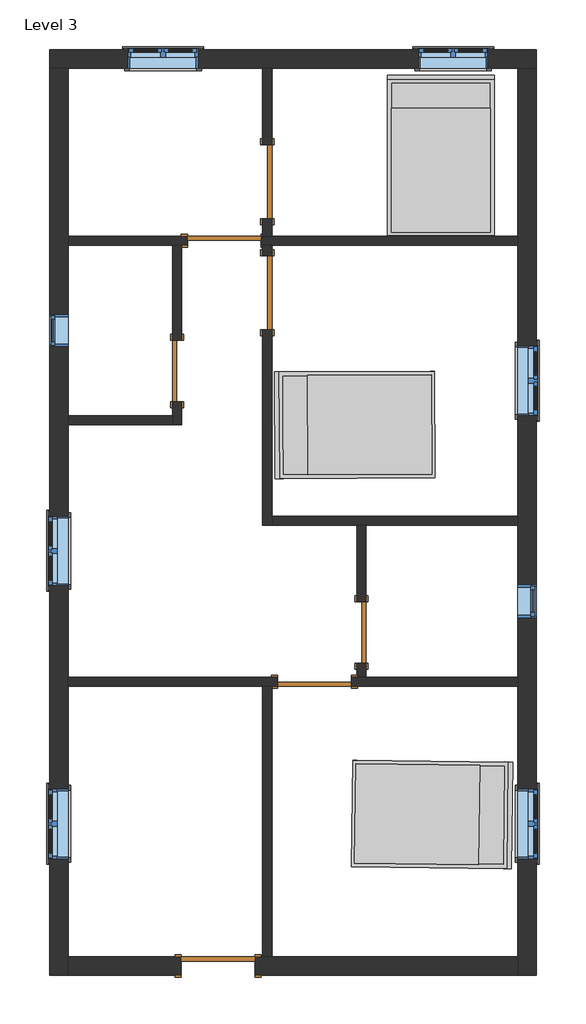
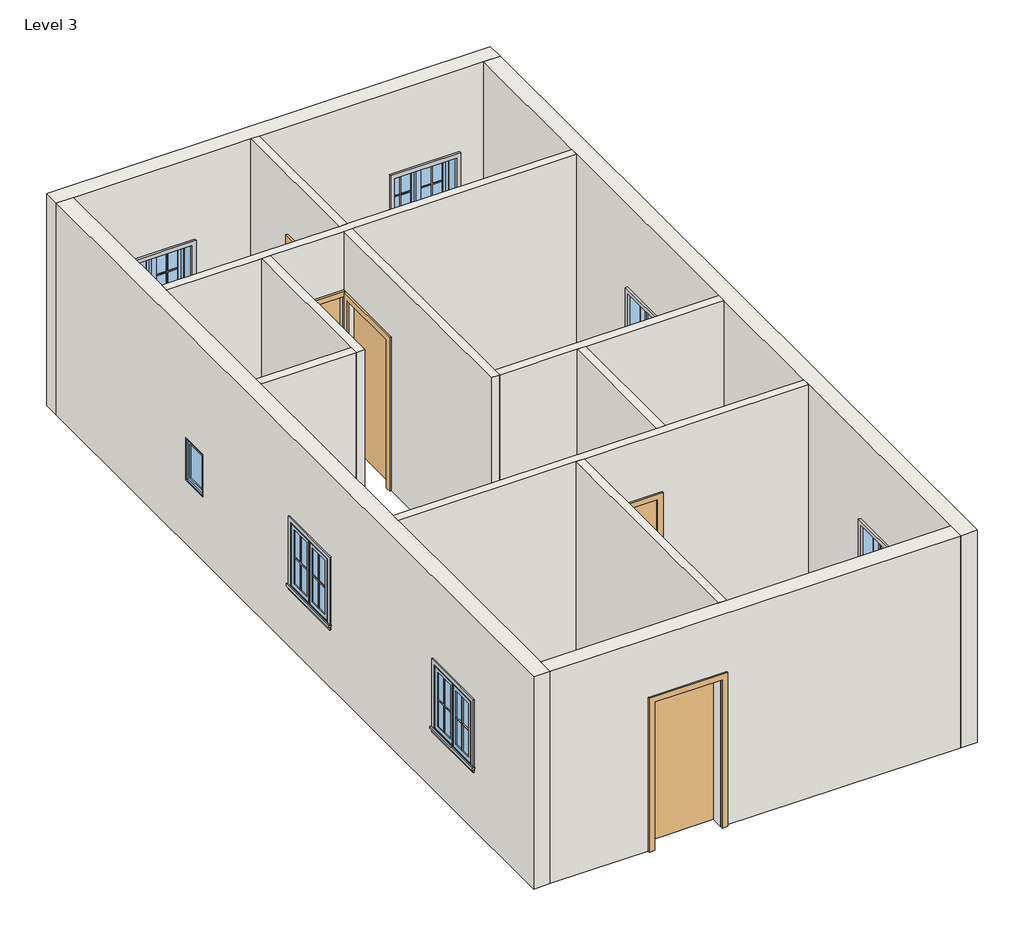
# One storey, incomplete: 24 proxies, 12 walls, 8 windows, 7 doors, 3 furniture elements.
"""IFC4 building model written with IfcOpenShell, lengths in millimetres."""

from ifc_helpers import new_model, si_unit, frame, origin, place, context, project, spatial, polyline, outline, extrude, faceted_brep, transform, mapped, element, save
from components import muntin_pattern_2x2_muntin_pattern_2x2_b3fe6957, muntin_pattern_2x2_muntin_pattern_2x2_3e0ecaf2, trim_window_exterior_flat_with_sill_41619996, trim_window_interior_flat_picture_frame_51c85655, door_d8f5dbb5, door_f2b275c1, door_e5f9f3c4, door_305aa2a5, door_0ca8825f, bed_17739_bed_17739_15c61121, window_aa618e30, window_339605e1

model = new_model("IFC4")

# Units and contexts
model_context = context("Model", 3, world=origin())
ifc_project = project(units=[si_unit("LENGTHUNIT", "METRE", prefix="MILLI")], contexts=[model_context])

# Site, building, storey
site = spatial("IfcSite", under=ifc_project)
building = spatial("IfcBuilding", under=site)
storey = spatial("IfcBuildingStorey", under=building, Name="Level 3", Elevation=3200.4)

# Proxies
placement = place(None, origin())
muntin_pattern_2x2_muntin_pattern_2x2_shape = muntin_pattern_2x2_muntin_pattern_2x2_b3fe6957(model_context)
element("IfcBuildingElementProxy", 1, Name="Muntin Pattern_2x2 : Muntin Pattern_2x2", ObjectType="Muntin Pattern_2x2 : Muntin Pattern_2x2", at=placement, inside=storey, context=model_context, shape_type="MappedRepresentation", body=[
    mapped(muntin_pattern_2x2_muntin_pattern_2x2_shape, transform((517.9959916, 6415.1185985, 4184.65), x_axis=(1.0, 0.0, 0.0), y_axis=(0.0, 1.0, 0.0), z_axis=(0.0, 0.0, 1.0))),
])
element("IfcBuildingElementProxy", 2, Name="Muntin Pattern_2x2 : Muntin Pattern_2x2", ObjectType="Muntin Pattern_2x2 : Muntin Pattern_2x2", at=placement, inside=storey, context=model_context, shape_type="MappedRepresentation", body=[
    mapped(muntin_pattern_2x2_muntin_pattern_2x2_shape, transform((-3079.2790084, 6415.1185985, 4184.65), x_axis=(1.0, 0.0, 0.0), y_axis=(0.0, 1.0, 0.0), z_axis=(0.0, 0.0, 1.0))),
])
element("IfcBuildingElementProxy", 3, Name="Muntin Pattern_2x2 : Muntin Pattern_2x2", ObjectType="Muntin Pattern_2x2 : Muntin Pattern_2x2", at=placement, inside=storey, context=model_context, shape_type="MappedRepresentation", body=[
    mapped(muntin_pattern_2x2_muntin_pattern_2x2_shape, transform((1751.4834916, 2536.8560985, 4184.65), x_axis=(0.0, -1.0, 0.0), y_axis=(1.0, 0.0, 0.0), z_axis=(0.0, 0.0, 1.0))),
])
element("IfcBuildingElementProxy", 4, Name="Muntin Pattern_2x2 : Muntin Pattern_2x2", ObjectType="Muntin Pattern_2x2 : Muntin Pattern_2x2", at=placement, inside=storey, context=model_context, shape_type="MappedRepresentation", body=[
    mapped(muntin_pattern_2x2_muntin_pattern_2x2_shape, transform((-4261.9665084, 0.0310985, 4184.65), x_axis=(0.0, 1.0, 0.0), y_axis=(-1.0, 0.0, 0.0), z_axis=(0.0, 0.0, 1.0))),
])
element("IfcBuildingElementProxy", 5, Name="Muntin Pattern_2x2 : Muntin Pattern_2x2", ObjectType="Muntin Pattern_2x2 : Muntin Pattern_2x2", at=placement, inside=storey, context=model_context, shape_type="MappedRepresentation", body=[
    mapped(muntin_pattern_2x2_muntin_pattern_2x2_shape, transform((-4261.9665084, -3381.3439015, 4184.65), x_axis=(0.0, 1.0, 0.0), y_axis=(-1.0, 0.0, 0.0), z_axis=(0.0, 0.0, 1.0))),
])
element("IfcBuildingElementProxy", 6, Name="Muntin Pattern_2x2 : Muntin Pattern_2x2", ObjectType="Muntin Pattern_2x2 : Muntin Pattern_2x2", at=placement, inside=storey, context=model_context, shape_type="MappedRepresentation", body=[
    mapped(muntin_pattern_2x2_muntin_pattern_2x2_shape, transform((1751.4834916, -2952.7189015, 4184.65), x_axis=(0.0, -1.0, 0.0), y_axis=(1.0, 0.0, 0.0), z_axis=(0.0, 0.0, 1.0))),
])
muntin_pattern_2x2_muntin_pattern_2x2_2_shape = muntin_pattern_2x2_muntin_pattern_2x2_3e0ecaf2(model_context)
element("IfcBuildingElementProxy", 7, Name="Muntin Pattern_2x2 : Muntin Pattern_2x2", ObjectType="Muntin Pattern_2x2 : Muntin Pattern_2x2", at=placement, inside=storey, context=model_context, shape_type="MappedRepresentation", body=[
    mapped(muntin_pattern_2x2_muntin_pattern_2x2_2_shape, transform((946.6209916, 6415.1185985, 4184.65), x_axis=(-1.0, 0.0, 0.0), y_axis=(0.0, -1.0, 0.0), z_axis=(0.0, 0.0, 1.0))),
])
element("IfcBuildingElementProxy", 8, Name="Muntin Pattern_2x2 : Muntin Pattern_2x2", ObjectType="Muntin Pattern_2x2 : Muntin Pattern_2x2", at=placement, inside=storey, context=model_context, shape_type="MappedRepresentation", body=[
    mapped(muntin_pattern_2x2_muntin_pattern_2x2_2_shape, transform((-2650.6540084, 6415.1185985, 4184.65), x_axis=(-1.0, 0.0, 0.0), y_axis=(0.0, -1.0, 0.0), z_axis=(0.0, 0.0, 1.0))),
])
element("IfcBuildingElementProxy", 9, Name="Muntin Pattern_2x2 : Muntin Pattern_2x2", ObjectType="Muntin Pattern_2x2 : Muntin Pattern_2x2", at=placement, inside=storey, context=model_context, shape_type="MappedRepresentation", body=[
    mapped(muntin_pattern_2x2_muntin_pattern_2x2_2_shape, transform((1751.4834916, 2108.2310985, 4184.65), x_axis=(0.0, 1.0, 0.0), y_axis=(-1.0, 0.0, 0.0), z_axis=(0.0, 0.0, 1.0))),
])
element("IfcBuildingElementProxy", 10, Name="Muntin Pattern_2x2 : Muntin Pattern_2x2", ObjectType="Muntin Pattern_2x2 : Muntin Pattern_2x2", at=placement, inside=storey, context=model_context, shape_type="MappedRepresentation", body=[
    mapped(muntin_pattern_2x2_muntin_pattern_2x2_2_shape, transform((-4261.9665084, 428.6560985, 4184.65), x_axis=(0.0, -1.0, 0.0), y_axis=(1.0, 0.0, 0.0), z_axis=(0.0, 0.0, 1.0))),
])
element("IfcBuildingElementProxy", 11, Name="Muntin Pattern_2x2 : Muntin Pattern_2x2", ObjectType="Muntin Pattern_2x2 : Muntin Pattern_2x2", at=placement, inside=storey, context=model_context, shape_type="MappedRepresentation", body=[
    mapped(muntin_pattern_2x2_muntin_pattern_2x2_2_shape, transform((-4261.9665084, -2952.7189015, 4184.65), x_axis=(0.0, -1.0, 0.0), y_axis=(1.0, 0.0, 0.0), z_axis=(0.0, 0.0, 1.0))),
])
element("IfcBuildingElementProxy", 12, Name="Muntin Pattern_2x2 : Muntin Pattern_2x2", ObjectType="Muntin Pattern_2x2 : Muntin Pattern_2x2", at=placement, inside=storey, context=model_context, shape_type="MappedRepresentation", body=[
    mapped(muntin_pattern_2x2_muntin_pattern_2x2_2_shape, transform((1751.4834916, -3381.3439015, 4184.65), x_axis=(0.0, 1.0, 0.0), y_axis=(-1.0, 0.0, 0.0), z_axis=(0.0, 0.0, 1.0))),
])
trim_window_exterior_flat_with_sill_shape = trim_window_exterior_flat_with_sill_41619996(model_context)
element("IfcBuildingElementProxy", 13, Name="Trim-Window-Exterior-Flat : with Sill", ObjectType="Trim-Window-Exterior-Flat : with Sill", at=placement, inside=storey, context=model_context, shape_type="MappedRepresentation", body=[
    mapped(trim_window_exterior_flat_with_sill_shape, transform((732.3084916, 6424.6435985, 5029.2), x_axis=(-1.0, 0.0, 0.0), y_axis=(0.0, 0.0, 1.0), z_axis=(0.0, 1.0, 0.0))),
])
element("IfcBuildingElementProxy", 14, Name="Trim-Window-Exterior-Flat : with Sill", ObjectType="Trim-Window-Exterior-Flat : with Sill", at=placement, inside=storey, context=model_context, shape_type="MappedRepresentation", body=[
    mapped(trim_window_exterior_flat_with_sill_shape, transform((-2864.9665084, 6424.6435985, 5029.2), x_axis=(-1.0, 0.0, 0.0), y_axis=(0.0, 0.0, 1.0), z_axis=(0.0, 1.0, 0.0))),
])
element("IfcBuildingElementProxy", 15, Name="Trim-Window-Exterior-Flat : with Sill", ObjectType="Trim-Window-Exterior-Flat : with Sill", at=placement, inside=storey, context=model_context, shape_type="MappedRepresentation", body=[
    mapped(trim_window_exterior_flat_with_sill_shape, transform((1761.0084916, 2322.5435985, 5029.2), x_axis=(0.0, 1.0, 0.0), y_axis=(0.0, 0.0, 1.0), z_axis=(1.0, 0.0, 0.0))),
])
element("IfcBuildingElementProxy", 16, Name="Trim-Window-Exterior-Flat : with Sill", ObjectType="Trim-Window-Exterior-Flat : with Sill", at=placement, inside=storey, context=model_context, shape_type="MappedRepresentation", body=[
    mapped(trim_window_exterior_flat_with_sill_shape, transform((-4271.4915084, 214.3435985, 5029.2), x_axis=(0.0, -1.0, 0.0), y_axis=(0.0, 0.0, 1.0), z_axis=(-1.0, 0.0, 0.0))),
])
element("IfcBuildingElementProxy", 17, Name="Trim-Window-Exterior-Flat : with Sill", ObjectType="Trim-Window-Exterior-Flat : with Sill", at=placement, inside=storey, context=model_context, shape_type="MappedRepresentation", body=[
    mapped(trim_window_exterior_flat_with_sill_shape, transform((-4271.4915084, -3167.0314015, 5029.2), x_axis=(0.0, -1.0, 0.0), y_axis=(0.0, 0.0, 1.0), z_axis=(-1.0, 0.0, 0.0))),
])
element("IfcBuildingElementProxy", 18, Name="Trim-Window-Exterior-Flat : with Sill", ObjectType="Trim-Window-Exterior-Flat : with Sill", at=placement, inside=storey, context=model_context, shape_type="MappedRepresentation", body=[
    mapped(trim_window_exterior_flat_with_sill_shape, transform((1761.0084916, -3167.0314015, 5029.2), x_axis=(0.0, 1.0, 0.0), y_axis=(0.0, 0.0, 1.0), z_axis=(1.0, 0.0, 0.0))),
])
trim_window_interior_flat_picture_frame_shape = trim_window_interior_flat_picture_frame_51c85655(model_context)
element("IfcBuildingElementProxy", 19, Name="Trim-Window-Interior-Flat : Picture Frame", ObjectType="Trim-Window-Interior-Flat : Picture Frame", at=placement, inside=storey, context=model_context, shape_type="MappedRepresentation", body=[
    mapped(trim_window_interior_flat_picture_frame_shape, transform((732.3084916, 6196.0435985, 5029.2), x_axis=(1.0, 0.0, 0.0), y_axis=(0.0, 0.0, 1.0), z_axis=(0.0, -1.0, 0.0))),
])
element("IfcBuildingElementProxy", 20, Name="Trim-Window-Interior-Flat : Picture Frame", ObjectType="Trim-Window-Interior-Flat : Picture Frame", at=placement, inside=storey, context=model_context, shape_type="MappedRepresentation", body=[
    mapped(trim_window_interior_flat_picture_frame_shape, transform((-2864.9665084, 6196.0435985, 5029.2), x_axis=(1.0, 0.0, 0.0), y_axis=(0.0, 0.0, 1.0), z_axis=(0.0, -1.0, 0.0))),
])
element("IfcBuildingElementProxy", 21, Name="Trim-Window-Interior-Flat : Picture Frame", ObjectType="Trim-Window-Interior-Flat : Picture Frame", at=placement, inside=storey, context=model_context, shape_type="MappedRepresentation", body=[
    mapped(trim_window_interior_flat_picture_frame_shape, transform((1532.4084916, 2322.5435985, 5029.2), x_axis=(0.0, -1.0, 0.0), y_axis=(0.0, 0.0, 1.0), z_axis=(-1.0, 0.0, 0.0))),
])
element("IfcBuildingElementProxy", 22, Name="Trim-Window-Interior-Flat : Picture Frame", ObjectType="Trim-Window-Interior-Flat : Picture Frame", at=placement, inside=storey, context=model_context, shape_type="MappedRepresentation", body=[
    mapped(trim_window_interior_flat_picture_frame_shape, transform((-4042.8915084, 214.3435985, 5029.2), x_axis=(0.0, 1.0, 0.0), y_axis=(0.0, 0.0, 1.0), z_axis=(1.0, 0.0, 0.0))),
])
element("IfcBuildingElementProxy", 23, Name="Trim-Window-Interior-Flat : Picture Frame", ObjectType="Trim-Window-Interior-Flat : Picture Frame", at=placement, inside=storey, context=model_context, shape_type="MappedRepresentation", body=[
    mapped(trim_window_interior_flat_picture_frame_shape, transform((-4042.8915084, -3167.0314015, 5029.2), x_axis=(0.0, 1.0, 0.0), y_axis=(0.0, 0.0, 1.0), z_axis=(1.0, 0.0, 0.0))),
])
element("IfcBuildingElementProxy", 24, Name="Trim-Window-Interior-Flat : Picture Frame", ObjectType="Trim-Window-Interior-Flat : Picture Frame", at=placement, inside=storey, context=model_context, shape_type="MappedRepresentation", body=[
    mapped(trim_window_interior_flat_picture_frame_shape, transform((1532.4084916, -3167.0314015, 5029.2), x_axis=(0.0, -1.0, 0.0), y_axis=(0.0, 0.0, 1.0), z_axis=(-1.0, 0.0, 0.0))),
])

# Doors
door_shape = door_d8f5dbb5(model_context)
element("IfcDoor", 25, ObjectType="Single-Flush : 30\" x 80\"", at=placement, inside=storey, context=model_context, shape_type="MappedRepresentation", body=[
    mapped(door_shape, transform((-404.3415084, -795.3064015, 3200.4), x_axis=(0.0, -1.0, 0.0), y_axis=(1.0, 0.0, 0.0), z_axis=(0.0, 0.0, 1.0))),
])
door_2_shape = door_f2b275c1(model_context)
element("IfcDoor", 26, ObjectType="Single-Flush : 30\" x 80\"", at=placement, inside=storey, context=model_context, shape_type="MappedRepresentation", body=[
    mapped(door_2_shape, transform((-2690.3415084, 2443.1935985, 3200.4), x_axis=(0.0, -1.0, 0.0), y_axis=(1.0, 0.0, 0.0), z_axis=(0.0, 0.0, 1.0))),
])
door_3_shape = door_e5f9f3c4(model_context)
element("IfcDoor", 27, ObjectType="Single-Flush : 36\" x 84\"", at=placement, inside=storey, context=model_context, shape_type="MappedRepresentation", body=[
    mapped(door_3_shape, transform((-2106.1415084, 4056.0935985, 3200.4), x_axis=(1.0, 0.0, 0.0), y_axis=(0.0, 1.0, 0.0), z_axis=(0.0, 0.0, 1.0))),
])
element("IfcDoor", 28, ObjectType="Single-Flush : 36\" x 84\"", at=placement, inside=storey, context=model_context, shape_type="MappedRepresentation", body=[
    mapped(door_3_shape, transform((-1572.7415084, 4786.3435985, 3200.4), x_axis=(0.0, -1.0, 0.0), y_axis=(1.0, 0.0, 0.0), z_axis=(0.0, 0.0, 1.0))),
])
element("IfcDoor", 29, ObjectType="Single-Flush : 36\" x 84\"", at=placement, inside=storey, context=model_context, shape_type="MappedRepresentation", body=[
    mapped(door_3_shape, transform((-988.5415084, -1404.9064015, 3200.4), x_axis=(-1.0, 0.0, 0.0), y_axis=(0.0, -1.0, 0.0), z_axis=(0.0, 0.0, 1.0))),
])
door_4_shape = door_305aa2a5(model_context)
element("IfcDoor", 30, ObjectType="Single-Flush : 36\" x 84\"", at=placement, inside=storey, context=model_context, shape_type="MappedRepresentation", body=[
    mapped(door_4_shape, transform((-1572.7415084, 3414.7435985, 3200.4), x_axis=(0.0, 1.0, 0.0), y_axis=(-1.0, 0.0, 0.0), z_axis=(0.0, 0.0, 1.0))),
])
door_5_shape = door_0ca8825f(model_context)
element("IfcDoor", 31, ObjectType="Single-Flush : 36\" x 84\"", at=placement, inside=storey, context=model_context, shape_type="MappedRepresentation", body=[
    mapped(door_5_shape, transform((-2182.3415084, -4929.1564015, 3200.4), x_axis=(1.0, 0.0, 0.0), y_axis=(0.0, 1.0, 0.0), z_axis=(0.0, 0.0, 1.0))),
])

# Furniture
bed_17739_bed_17739_shape = bed_17739_bed_17739_15c61121(model_context)
element("IfcFurniture", 32, ObjectType="Bed_17739 : Bed_17739", at=placement, inside=storey, context=model_context, shape_type="MappedRepresentation", body=[
    mapped(bed_17739_bed_17739_shape, transform((579.9084916, 5091.1435985, 3200.4), x_axis=(1.0, 0.0, 0.0), y_axis=(0.0, 1.0, 0.0), z_axis=(0.0, 0.0, 1.0))),
])
element("IfcFurniture", 33, ObjectType="Bed_17739 : Bed_17739", at=placement, inside=storey, context=model_context, shape_type="MappedRepresentation", body=[
    mapped(bed_17739_bed_17739_shape, transform((-461.4915084, 1776.4435985, 3200.4), x_axis=(-0.00529598194226197, 0.9999859761893001, 0.0), y_axis=(-0.9999859761893001, -0.00529598194226197, 0.0), z_axis=(0.0, 0.0, 1.0))),
])
element("IfcFurniture", 34, ObjectType="Bed_17739 : Bed_17739", at=placement, inside=storey, context=model_context, shape_type="MappedRepresentation", body=[
    mapped(bed_17739_bed_17739_shape, transform((445.2457081, -3048.1973462, 3200.4), x_axis=(-0.012781947661401841, -0.9999183075701641, 0.0), y_axis=(0.9999183075701641, -0.012781947661401841, 0.0), z_axis=(0.0, 0.0, 1.0))),
])

# Walls
element("IfcWall", 35, ObjectType="WALL4.5\"", at=placement, inside=storey, context=model_context, shape_type="Brep", body=[
    faceted_brep([(-1648.9415084, 3998.9435985, 5334.0), (-1648.9415084, 3998.9435985, 3200.4), (-1629.8915084, 3998.9435985, 3200.4), (-1515.5915084, 3998.9435985, 3200.4), (1532.4084916, 3998.9435985, 3200.4), (1532.4084916, 3998.9435985, 6248.4), (-1515.5915084, 3998.9435985, 6248.4), (-1629.8915084, 3998.9435985, 6248.4), (-2633.1915084, 3998.9435985, 6248.4), (-2747.4915084, 3998.9435985, 6248.4), (-4042.8915084, 3998.9435985, 6248.4), (-4042.8915084, 3998.9435985, 3200.4), (-2747.4915084, 3998.9435985, 3200.4), (-2633.1915084, 3998.9435985, 3200.4), (-2563.3415084, 3998.9435985, 3200.4), (-2563.3415084, 3998.9435985, 5334.0), (1532.4084916, 4113.2435985, 3200.4), (-1515.5915084, 4113.2435985, 3200.4), (-1629.8915084, 4113.2435985, 3200.4), (-1648.9415084, 4113.2435985, 3200.4), (-1648.9415084, 4113.2435985, 5334.0), (-2563.3415084, 4113.2435985, 5334.0), (-2563.3415084, 4113.2435985, 3200.4), (-4042.8915084, 4113.2435985, 3200.4), (-4042.8915084, 4113.2435985, 6248.4), (-1629.8915084, 4113.2435985, 6248.4), (-1515.5915084, 4113.2435985, 6248.4), (1532.4084916, 4113.2435985, 6248.4)], [[[0, 1, 2, 3, 4, 5, 6, 7, 8, 9, 10, 11, 12, 13, 14, 15]], [[16, 17, 18, 19, 20, 21, 22, 23, 24, 25, 26, 27]], [[4, 3, 2, 1, 19, 18, 17, 16]], [[14, 13, 12, 11, 23, 22]], [[5, 4, 16, 27]], [[11, 10, 24, 23]], [[20, 19, 1, 0]], [[21, 20, 0, 15]], [[22, 21, 15, 14]], [[10, 9, 8, 7, 6, 5, 27, 26, 25, 24]]]),
])
element("IfcWall", 36, ObjectType="WALL4.5\"", at=placement, inside=storey, context=model_context, shape_type="Brep", body=[
    faceted_brep([(-1629.8915084, 6196.0435985, 6248.4), (-1629.8915084, 6196.0435985, 3200.4), (-1629.8915084, 5243.5435985, 3200.4), (-1629.8915084, 5243.5435985, 5334.0), (-1629.8915084, 4329.1435985, 5334.0), (-1629.8915084, 4329.1435985, 3200.4), (-1629.8915084, 4113.2435985, 3200.4), (-1629.8915084, 4113.2435985, 6248.4), (-1515.5915084, 6196.0435985, 3200.4), (-1515.5915084, 6196.0435985, 6248.4), (-1515.5915084, 4113.2435985, 6248.4), (-1515.5915084, 4113.2435985, 3200.4), (-1515.5915084, 4329.1435985, 3200.4), (-1515.5915084, 4329.1435985, 5334.0), (-1515.5915084, 5243.5435985, 5334.0), (-1515.5915084, 5243.5435985, 3200.4)], [[[0, 1, 2, 3, 4, 5, 6, 7]], [[8, 9, 10, 11, 12, 13, 14, 15]], [[1, 8, 15, 2]], [[5, 12, 11, 6]], [[1, 0, 9, 8]], [[7, 6, 11, 10]], [[13, 12, 5, 4]], [[14, 13, 4, 3]], [[15, 14, 3, 2]], [[9, 0, 7, 10]]]),
    faceted_brep([(-1629.8915084, 531.8435985, 3200.4), (-1629.8915084, 531.8435985, 6248.4), (-1629.8915084, 3998.9435985, 6248.4), (-1629.8915084, 3998.9435985, 3200.4), (-1629.8915084, 3871.9435985, 3200.4), (-1629.8915084, 3871.9435985, 5334.0), (-1629.8915084, 2957.5435985, 5334.0), (-1629.8915084, 2957.5435985, 3200.4), (-1515.5915084, 531.8435985, 6248.4), (-1515.5915084, 531.8435985, 3200.4), (-1515.5915084, 646.1435985, 3200.4), (-1515.5915084, 2957.5435985, 3200.4), (-1515.5915084, 2957.5435985, 5334.0), (-1515.5915084, 3871.9435985, 5334.0), (-1515.5915084, 3871.9435985, 3200.4), (-1515.5915084, 3998.9435985, 3200.4), (-1515.5915084, 3998.9435985, 6248.4), (-1515.5915084, 646.1435985, 6248.4)], [[[0, 1, 2, 3, 4, 5, 6, 7]], [[8, 9, 10, 11, 12, 13, 14, 15, 16, 17]], [[9, 0, 7, 11, 10]], [[14, 4, 3, 15]], [[3, 2, 16, 15]], [[1, 0, 9, 8]], [[5, 4, 14, 13]], [[6, 5, 13, 12]], [[7, 6, 12, 11]], [[1, 8, 17, 16, 2]]]),
])
element("IfcWall", 37, ObjectType="WALL4.5\"", at=placement, inside=storey, context=model_context, shape_type="Brep", body=[
    faceted_brep([(-1515.5915084, 531.8435985, 3200.4), (-461.4915084, 531.8435985, 3200.4), (-347.1915084, 531.8435985, 3200.4), (1532.4084916, 531.8435985, 3200.4), (1532.4084916, 531.8435985, 6248.4), (-347.1915084, 531.8435985, 6248.4), (-461.4915084, 531.8435985, 6248.4), (-1515.5915084, 531.8435985, 6248.4), (-1515.5915084, 646.1435985, 3200.4), (-1515.5915084, 646.1435985, 6248.4), (1532.4084916, 646.1435985, 6248.4), (1532.4084916, 646.1435985, 3200.4)], [[[0, 1, 2, 3, 4, 5, 6, 7]], [[8, 9, 10, 11]], [[3, 2, 1, 0, 8, 11]], [[0, 7, 9, 8]], [[4, 3, 11, 10]], [[7, 6, 5, 4, 10, 9]]]),
])
element("IfcWall", 38, ObjectType="WALL4.5\"", at=placement, inside=storey, context=model_context, shape_type="Brep", body=[
    faceted_brep([(-2747.4915084, 2062.1935985, 5232.4), (-2747.4915084, 2062.1935985, 3200.4), (-2747.4915084, 1890.7435985, 3200.4), (-2747.4915084, 1776.4435985, 3200.4), (-2747.4915084, 1776.4435985, 6248.4), (-2747.4915084, 1890.7435985, 6248.4), (-2747.4915084, 3998.9435985, 6248.4), (-2747.4915084, 3998.9435985, 3200.4), (-2747.4915084, 2824.1935985, 3200.4), (-2747.4915084, 2824.1935985, 5232.4), (-2633.1915084, 1776.4435985, 3200.4), (-2633.1915084, 2062.1935985, 3200.4), (-2633.1915084, 2062.1935985, 5232.4), (-2633.1915084, 2824.1935985, 5232.4), (-2633.1915084, 2824.1935985, 3200.4), (-2633.1915084, 3998.9435985, 3200.4), (-2633.1915084, 3998.9435985, 6248.4), (-2633.1915084, 1776.4435985, 6248.4)], [[[0, 1, 2, 3, 4, 5, 6, 7, 8, 9]], [[10, 11, 12, 13, 14, 15, 16, 17]], [[8, 7, 15, 14]], [[3, 2, 1, 11, 10]], [[7, 6, 16, 15]], [[4, 3, 10, 17]], [[12, 11, 1, 0]], [[13, 12, 0, 9]], [[14, 13, 9, 8]], [[6, 5, 4, 17, 16]]]),
])
element("IfcWall", 39, ObjectType="WALL4.5\"", at=placement, inside=storey, context=model_context, shape_type="SweptSolid", body=[
    extrude(outline(polyline([(-2747.4915084, 1776.4435985), (-4042.8915084, 1776.4435985), (-4042.8915084, 1890.7435985), (-2747.4915084, 1890.7435985), (-2747.4915084, 1776.4435985)])), frame((0.0, 0.0, 3200.4), z_axis=(0.0, 0.0, 1.0), x_axis=(1.0, 0.0, 0.0)), (0.0, 0.0, 1.0), 3048.0),
])
element("IfcWall", 40, ObjectType="WALL4.5\"", at=placement, inside=storey, context=model_context, shape_type="SweptSolid", body=[
    extrude(outline(polyline([(-1176.3064015, 5232.4), (-1176.3064015, 3200.4), (-1347.7564015, 3200.4), (-1347.7564015, 6248.4), (531.8435985, 6248.4), (531.8435985, 3200.4), (-414.3064015, 3200.4), (-414.3064015, 5232.4), (-1176.3064015, 5232.4)])), frame((-461.4915084, 0.0, 0.0), z_axis=(1.0, 0.0, 0.0), x_axis=(0.0, 1.0, 0.0)), (0.0, 0.0, 1.0), 114.3),
])
element("IfcWall", 41, ObjectType="WALL4.5\"", at=placement, inside=storey, context=model_context, shape_type="Brep", body=[
    faceted_brep([(-4042.8915084, -1462.0564015, 3200.4), (-1629.8915084, -1462.0564015, 3200.4), (-1515.5915084, -1462.0564015, 3200.4), (-1445.7415084, -1462.0564015, 3200.4), (-1445.7415084, -1462.0564015, 5334.0), (-531.3415084, -1462.0564015, 5334.0), (-531.3415084, -1462.0564015, 3200.4), (1532.4084916, -1462.0564015, 3200.4), (1532.4084916, -1462.0564015, 6248.4), (-1515.5915084, -1462.0564015, 6248.4), (-1629.8915084, -1462.0564015, 6248.4), (-4042.8915084, -1462.0564015, 6248.4), (-1445.7415084, -1347.7564015, 5334.0), (-1445.7415084, -1347.7564015, 3200.4), (-4042.8915084, -1347.7564015, 3200.4), (-4042.8915084, -1347.7564015, 6248.4), (-461.4915084, -1347.7564015, 6248.4), (-347.1915084, -1347.7564015, 6248.4), (1532.4084916, -1347.7564015, 6248.4), (1532.4084916, -1347.7564015, 3200.4), (-347.1915084, -1347.7564015, 3200.4), (-461.4915084, -1347.7564015, 3200.4), (-531.3415084, -1347.7564015, 3200.4), (-531.3415084, -1347.7564015, 5334.0)], [[[0, 1, 2, 3, 4, 5, 6, 7, 8, 9, 10, 11]], [[12, 13, 14, 15, 16, 17, 18, 19, 20, 21, 22, 23]], [[14, 13, 3, 2, 1, 0]], [[22, 21, 20, 19, 7, 6]], [[8, 7, 19, 18]], [[0, 11, 15, 14]], [[4, 3, 13, 12]], [[5, 4, 12, 23]], [[6, 5, 23, 22]], [[11, 10, 9, 8, 18, 17, 16, 15]]]),
])
element("IfcWall", 42, ObjectType="WALL4.5\"", at=placement, inside=storey, context=model_context, shape_type="SweptSolid", body=[
    extrude(outline(polyline([(-1629.8915084, -4814.8564015), (-1629.8915084, -1462.0564015), (-1515.5915084, -1462.0564015), (-1515.5915084, -4814.8564015), (-1629.8915084, -4814.8564015)])), frame((0.0, 0.0, 3200.4), z_axis=(0.0, 0.0, 1.0), x_axis=(1.0, 0.0, 0.0)), (0.0, 0.0, 1.0), 3048.0),
])
element("IfcWall", 43, ObjectType="WALL9\"", at=placement, inside=storey, context=model_context, shape_type="Brep", body=[
    faceted_brep([(-4271.4915084, 6196.0435985, 3200.4), (-4042.8915084, 6196.0435985, 3200.4), (-1629.8915084, 6196.0435985, 3200.4), (-1515.5915084, 6196.0435985, 3200.4), (1532.4084916, 6196.0435985, 3200.4), (1761.0084916, 6196.0435985, 3200.4), (1761.0084916, 6196.0435985, 6248.4), (1532.4084916, 6196.0435985, 6248.4), (-1515.5915084, 6196.0435985, 6248.4), (-1629.8915084, 6196.0435985, 6248.4), (-4042.8915084, 6196.0435985, 6248.4), (-4271.4915084, 6196.0435985, 6248.4), (1164.1084916, 6196.0435985, 5029.2), (1164.1084916, 6196.0435985, 4114.8), (300.5084916, 6196.0435985, 4114.8), (300.5084916, 6196.0435985, 5029.2), (-2433.1665084, 6196.0435985, 5029.2), (-2433.1665084, 6196.0435985, 4114.8), (-3296.7665084, 6196.0435985, 4114.8), (-3296.7665084, 6196.0435985, 5029.2), (-4271.4915084, 6424.6435985, 3200.4), (-4271.4915084, 6424.6435985, 6248.4), (1761.0084916, 6424.6435985, 6248.4), (1761.0084916, 6424.6435985, 3200.4), (1164.1084916, 6424.6435985, 5029.2), (300.5084916, 6424.6435985, 5029.2), (300.5084916, 6424.6435985, 4114.8), (1164.1084916, 6424.6435985, 4114.8), (-2433.1665084, 6424.6435985, 5029.2), (-3296.7665084, 6424.6435985, 5029.2), (-3296.7665084, 6424.6435985, 4114.8), (-2433.1665084, 6424.6435985, 4114.8)], [[[0, 1, 2, 3, 4, 5, 6, 7, 8, 9, 10, 11], [12, 13, 14, 15], [16, 17, 18, 19]], [[20, 21, 22, 23], [24, 25, 26, 27], [28, 29, 30, 31]], [[5, 4, 3, 2, 1, 0, 20, 23]], [[6, 5, 23, 22]], [[0, 11, 21, 20]], [[13, 12, 24, 27]], [[14, 13, 27, 26]], [[15, 14, 26, 25]], [[12, 15, 25, 24]], [[17, 16, 28, 31]], [[18, 17, 31, 30]], [[19, 18, 30, 29]], [[16, 19, 29, 28]], [[11, 10, 9, 8, 7, 6, 22, 21]]]),
])
element("IfcWall", 44, ObjectType="WALL9\"", at=placement, inside=storey, context=model_context, shape_type="Brep", body=[
    faceted_brep([(1532.4084916, 6196.0435985, 3200.4), (1532.4084916, 4113.2435985, 3200.4), (1532.4084916, 3998.9435985, 3200.4), (1532.4084916, 646.1435985, 3200.4), (1532.4084916, 531.8435985, 3200.4), (1532.4084916, -1347.7564015, 3200.4), (1532.4084916, -1462.0564015, 3200.4), (1532.4084916, -4814.8564015, 3200.4), (1532.4084916, -5043.4564015, 3200.4), (1532.4084916, -5043.4564015, 6248.4), (1532.4084916, -4814.8564015, 6248.4), (1532.4084916, -1462.0564015, 6248.4), (1532.4084916, -1347.7564015, 6248.4), (1532.4084916, 531.8435985, 6248.4), (1532.4084916, 646.1435985, 6248.4), (1532.4084916, 3998.9435985, 6248.4), (1532.4084916, 4113.2435985, 6248.4), (1532.4084916, 6196.0435985, 6248.4), (1532.4084916, -611.1564015, 4724.4), (1532.4084916, -611.1564015, 4114.8), (1532.4084916, -204.7564015, 4114.8), (1532.4084916, -204.7564015, 4724.4), (1532.4084916, 1890.7435985, 5029.2), (1532.4084916, 1890.7435985, 4114.8), (1532.4084916, 2754.3435985, 4114.8), (1532.4084916, 2754.3435985, 5029.2), (1532.4084916, -3598.8314015, 5029.2), (1532.4084916, -3598.8314015, 4114.8), (1532.4084916, -2735.2314015, 4114.8), (1532.4084916, -2735.2314015, 5029.2), (1761.0084916, 6196.0435985, 3200.4), (1761.0084916, 6196.0435985, 6248.4), (1761.0084916, -5043.4564015, 6248.4), (1761.0084916, -5043.4564015, 3200.4), (1761.0084916, -611.1564015, 4724.4), (1761.0084916, -204.7564015, 4724.4), (1761.0084916, -204.7564015, 4114.8), (1761.0084916, -611.1564015, 4114.8), (1761.0084916, 1890.7435985, 5029.2), (1761.0084916, 2754.3435985, 5029.2), (1761.0084916, 2754.3435985, 4114.8), (1761.0084916, 1890.7435985, 4114.8), (1761.0084916, -3598.8314015, 5029.2), (1761.0084916, -2735.2314015, 5029.2), (1761.0084916, -2735.2314015, 4114.8), (1761.0084916, -3598.8314015, 4114.8)], [[[0, 1, 2, 3, 4, 5, 6, 7, 8, 9, 10, 11, 12, 13, 14, 15, 16, 17], [18, 19, 20, 21], [22, 23, 24, 25], [26, 27, 28, 29]], [[30, 31, 32, 33], [34, 35, 36, 37], [38, 39, 40, 41], [42, 43, 44, 45]], [[8, 7, 6, 5, 4, 3, 2, 1, 0, 30, 33]], [[0, 17, 31, 30]], [[9, 8, 33, 32]], [[19, 18, 34, 37]], [[20, 19, 37, 36]], [[21, 20, 36, 35]], [[18, 21, 35, 34]], [[23, 22, 38, 41]], [[24, 23, 41, 40]], [[25, 24, 40, 39]], [[22, 25, 39, 38]], [[27, 26, 42, 45]], [[28, 27, 45, 44]], [[29, 28, 44, 43]], [[26, 29, 43, 42]], [[17, 16, 15, 14, 13, 12, 11, 10, 9, 32, 31]]]),
])
element("IfcWall", 45, ObjectType="WALL9\"", at=placement, inside=storey, context=model_context, shape_type="Brep", body=[
    faceted_brep([(-4271.4915084, 6196.0435985, 3200.4), (-4271.4915084, -5043.4564015, 3200.4), (-4271.4915084, -5043.4564015, 6248.4), (-4271.4915084, 6196.0435985, 6248.4), (-4271.4915084, 3148.0435985, 4724.4), (-4271.4915084, 2741.6435985, 4724.4), (-4271.4915084, 2741.6435985, 4114.8), (-4271.4915084, 3148.0435985, 4114.8), (-4271.4915084, 646.1435985, 5029.2), (-4271.4915084, -217.4564015, 5029.2), (-4271.4915084, -217.4564015, 4114.8), (-4271.4915084, 646.1435985, 4114.8), (-4271.4915084, -2735.2314015, 5029.2), (-4271.4915084, -3598.8314015, 5029.2), (-4271.4915084, -3598.8314015, 4114.8), (-4271.4915084, -2735.2314015, 4114.8), (-4042.8915084, 6196.0435985, 3200.4), (-4042.8915084, 6196.0435985, 6248.4), (-4042.8915084, 4113.2435985, 6248.4), (-4042.8915084, 3998.9435985, 6248.4), (-4042.8915084, 1890.7435985, 6248.4), (-4042.8915084, 1776.4435985, 6248.4), (-4042.8915084, -1347.7564015, 6248.4), (-4042.8915084, -1462.0564015, 6248.4), (-4042.8915084, -4814.8564015, 6248.4), (-4042.8915084, -5043.4564015, 6248.4), (-4042.8915084, -5043.4564015, 3200.4), (-4042.8915084, -4814.8564015, 3200.4), (-4042.8915084, -1462.0564015, 3200.4), (-4042.8915084, -1347.7564015, 3200.4), (-4042.8915084, 1776.4435985, 3200.4), (-4042.8915084, 1890.7435985, 3200.4), (-4042.8915084, 3998.9435985, 3200.4), (-4042.8915084, 4113.2435985, 3200.4), (-4042.8915084, 3148.0435985, 4724.4), (-4042.8915084, 3148.0435985, 4114.8), (-4042.8915084, 2741.6435985, 4114.8), (-4042.8915084, 2741.6435985, 4724.4), (-4042.8915084, 646.1435985, 5029.2), (-4042.8915084, 646.1435985, 4114.8), (-4042.8915084, -217.4564015, 4114.8), (-4042.8915084, -217.4564015, 5029.2), (-4042.8915084, -2735.2314015, 5029.2), (-4042.8915084, -2735.2314015, 4114.8), (-4042.8915084, -3598.8314015, 4114.8), (-4042.8915084, -3598.8314015, 5029.2)], [[[0, 1, 2, 3], [4, 5, 6, 7], [8, 9, 10, 11], [12, 13, 14, 15]], [[16, 17, 18, 19, 20, 21, 22, 23, 24, 25, 26, 27, 28, 29, 30, 31, 32, 33], [34, 35, 36, 37], [38, 39, 40, 41], [42, 43, 44, 45]], [[1, 0, 16, 33, 32, 31, 30, 29, 28, 27, 26]], [[0, 3, 17, 16]], [[2, 1, 26, 25]], [[35, 34, 4, 7]], [[36, 35, 7, 6]], [[37, 36, 6, 5]], [[34, 37, 5, 4]], [[39, 38, 8, 11]], [[40, 39, 11, 10]], [[41, 40, 10, 9]], [[38, 41, 9, 8]], [[43, 42, 12, 15]], [[44, 43, 15, 14]], [[45, 44, 14, 13]], [[42, 45, 13, 12]], [[3, 2, 25, 24, 23, 22, 21, 20, 19, 18, 17]]]),
])
element("IfcWall", 46, ObjectType="WALL9\"", at=placement, inside=storey, context=model_context, shape_type="Brep", body=[
    faceted_brep([(-1725.1415084, -5043.4564015, 5334.0), (-1725.1415084, -5043.4564015, 3200.4), (1532.4084916, -5043.4564015, 3200.4), (1532.4084916, -5043.4564015, 6248.4), (-4042.8915084, -5043.4564015, 6248.4), (-4042.8915084, -5043.4564015, 3200.4), (-2639.5415084, -5043.4564015, 3200.4), (-2639.5415084, -5043.4564015, 5334.0), (1532.4084916, -4814.8564015, 3200.4), (-1515.5915084, -4814.8564015, 3200.4), (-1629.8915084, -4814.8564015, 3200.4), (-1725.1415084, -4814.8564015, 3200.4), (-1725.1415084, -4814.8564015, 5334.0), (-2639.5415084, -4814.8564015, 5334.0), (-2639.5415084, -4814.8564015, 3200.4), (-4042.8915084, -4814.8564015, 3200.4), (-4042.8915084, -4814.8564015, 6248.4), (-1629.8915084, -4814.8564015, 6248.4), (-1515.5915084, -4814.8564015, 6248.4), (1532.4084916, -4814.8564015, 6248.4)], [[[0, 1, 2, 3, 4, 5, 6, 7]], [[8, 9, 10, 11, 12, 13, 14, 15, 16, 17, 18, 19]], [[6, 5, 15, 14]], [[2, 1, 11, 10, 9, 8]], [[3, 2, 8, 19]], [[5, 4, 16, 15]], [[12, 11, 1, 0]], [[13, 12, 0, 7]], [[14, 13, 7, 6]], [[4, 3, 19, 18, 17, 16]]]),
])

# Windows
window_shape = window_aa618e30(model_context)
element("IfcWindow", 47, ObjectType="Fixed : 16\" x 24\"", at=placement, inside=storey, context=model_context, shape_type="MappedRepresentation", body=[
    mapped(window_shape, transform((1646.7084916, -446.0564015, 3200.4), x_axis=(0.0, -1.0, 0.0), y_axis=(1.0, 0.0, 0.0), z_axis=(0.0, 0.0, 1.0))),
])
element("IfcWindow", 48, ObjectType="Fixed : 16\" x 24\"", at=placement, inside=storey, context=model_context, shape_type="MappedRepresentation", body=[
    mapped(window_shape, transform((-4157.1915084, 2982.9435985, 3200.4), x_axis=(0.0, 1.0, 0.0), y_axis=(-1.0, 0.0, 0.0), z_axis=(0.0, 0.0, 1.0))),
])
window_2_shape = window_339605e1(model_context)
element("IfcWindow", 49, ObjectType="Window-Casement-Double : 34\" x 36\"", at=placement, inside=storey, context=model_context, shape_type="MappedRepresentation", body=[
    mapped(window_2_shape, transform((732.3084916, 6310.3435985, 3200.4), x_axis=(1.0, 0.0, 0.0), y_axis=(0.0, 1.0, 0.0), z_axis=(0.0, 0.0, 1.0))),
])
element("IfcWindow", 50, ObjectType="Window-Casement-Double : 34\" x 36\"", at=placement, inside=storey, context=model_context, shape_type="MappedRepresentation", body=[
    mapped(window_2_shape, transform((-2864.9665084, 6310.3435985, 3200.4), x_axis=(1.0, 0.0, 0.0), y_axis=(0.0, 1.0, 0.0), z_axis=(0.0, 0.0, 1.0))),
])
element("IfcWindow", 51, ObjectType="Window-Casement-Double : 34\" x 36\"", at=placement, inside=storey, context=model_context, shape_type="MappedRepresentation", body=[
    mapped(window_2_shape, transform((1646.7084916, 2322.5435985, 3200.4), x_axis=(0.0, -1.0, 0.0), y_axis=(1.0, 0.0, 0.0), z_axis=(0.0, 0.0, 1.0))),
])
element("IfcWindow", 52, ObjectType="Window-Casement-Double : 34\" x 36\"", at=placement, inside=storey, context=model_context, shape_type="MappedRepresentation", body=[
    mapped(window_2_shape, transform((-4157.1915084, 214.3435985, 3200.4), x_axis=(0.0, 1.0, 0.0), y_axis=(-1.0, 0.0, 0.0), z_axis=(0.0, 0.0, 1.0))),
])
element("IfcWindow", 53, ObjectType="Window-Casement-Double : 34\" x 36\"", at=placement, inside=storey, context=model_context, shape_type="MappedRepresentation", body=[
    mapped(window_2_shape, transform((-4157.1915084, -3167.0314015, 3200.4), x_axis=(0.0, 1.0, 0.0), y_axis=(-1.0, 0.0, 0.0), z_axis=(0.0, 0.0, 1.0))),
])
element("IfcWindow", 54, ObjectType="Window-Casement-Double : 34\" x 36\"", at=placement, inside=storey, context=model_context, shape_type="MappedRepresentation", body=[
    mapped(window_2_shape, transform((1646.7084916, -3167.0314015, 3200.4), x_axis=(0.0, -1.0, 0.0), y_axis=(1.0, 0.0, 0.0), z_axis=(0.0, 0.0, 1.0))),
])

save(model, "model.ifc")

# Revit data of these elements
# Type "Muntin Pattern_2x2 : Muntin Pattern_2x2"
#   Width [instance default] = 4' - 0"
#   Thickness = 0' - 0 1/2"
#   Height [instance default] = 4' - 0"
#   Distance = 0' - 0 3/4"
#   Interior Material [instance default] = none
#   Exterior Material [instance default] = none
#   Default Elevation = 0
# Type "Trim-Window-Exterior-Flat : with Sill"
#   Trim Width = 0' - 2 1/4"
#   Trim Thickness_Picture Frame = 0' - 1 1/4"
#   Trim Thickness_with Sill = 0' - 0 3/4"
#   Sill Thickness = 0' - 1 1/4"
#   Opening Width [instance default] = 2' - 0"
#   Opening Height [instance default] = 3' - 0"
#   Default Elevation = 4' - 0"
#   Sill = yes
#   Picture Frame = no
#   Trim Material [instance default] = none
# Type "Trim-Window-Interior-Flat : Picture Frame"
#   Trim Thickness_Picture Frame = 0' - 1 1/4"
#   Trim Width = 0' - 2 1/4"
#   Trim Thickness_with Sill = 0' - 0 3/4"
#   Sill Thickness = 0' - 1 1/4"
#   Opening Width [instance default] = 2' - 0"
#   Opening Height [instance default] = 3' - 0"
#   Default Elevation = 4' - 0"
#   Sill = no
#   Picture Frame = yes
#   Trim Material [instance default] = none
# Type "Single-Flush : 30\" x 80\""
#   Type Mark = "5"
#   Construction Type Id = "MDOOR"
#   Assembly Code = "C1020"
#   Analytic Construction = "Metal"
#   Thickness = 0' - 2"
#   Heat Transfer Coefficient (U) = 0.651978 BTU/(h·ft²·°F)
#   Height = 6' - 8"
#   Trim Projection Ext = 0' - 1"
#   Trim Projection Int = 0' - 1"
#   Trim Width = 0' - 3"
#   Width = 2' - 6"
#   Define Thermal Properties by = 1
#   Define Thermal Properties by = 1
#   Door Material = Door - Panel
#   Frame Material = Door - Frame
#   Visual Light Transmittance = 0
#   Solar Heat Gain Coefficient = 0
#   Function = (empty or 0)
#   Wall Closure = (empty or 0)
# Type "Single-Flush : 36\" x 84\""
#   Type Mark = "1"
#   Construction Type Id = "MDOOR"
#   Assembly Code = "C1020"
#   Analytic Construction = "Metal"
#   Thickness = 0' - 2"
#   Heat Transfer Coefficient (U) = 0.651978 BTU/(h·ft²·°F)
#   Height = 7' - 0"
#   Trim Projection Ext = 0' - 1"
#   Trim Projection Int = 0' - 1"
#   Trim Width = 0' - 3"
#   Width = 3' - 0"
#   Define Thermal Properties by = 1
#   Define Thermal Properties by = 1
#   Door Material = Door - Panel
#   Frame Material = Door - Frame
#   Visual Light Transmittance = 0
#   Solar Heat Gain Coefficient = 0
#   Function = (empty or 0)
#   Wall Closure = (empty or 0)
# Type "Bed_17739 : Bed_17739"
#   Default Elevation = 0
# Type "WALL4.5\""
#   Assembly Code = "B2010"
#   Layers, outside or top first: 0' - 4 1/2" no material (function 1)
# Type "WALL9\""
#   Assembly Code = "B2010"
#   Layers, outside or top first: 0' - 9" no material (function 1)
# Type "Fixed : 16\" x 24\""
#   Type Mark = "4"
#   Construction Type Id = "GSP4R"
#   Assembly Code = "B2020100"
#   Analytic Construction = "1/8 in Pilkington single glazing"
#   Visual Light Transmittance = 0.9
#   Solar Heat Gain Coefficient = 0.78
#   Heat Transfer Coefficient (U) = 0.6496 BTU/(h·ft²·°F)
#   Height = 2' - 0"
#   Default Sill Height = 3' - 0"
#   Width = 1' - 4"
#   Window Inset = 0' - 0 3/4"
#   Define Thermal Properties by = 1
#   Define Thermal Properties by = 1
#   Glass Pane Material = Glass
#   Sash Material = Sash
#   Wall Closure = (empty or 0)
# Type "Window-Casement-Double : 34\" x 36\""
#   Type Mark = "14"
#   Fire Rating = "0.5h"
#   Assembly Code = "B2020100"
#   Analytic Construction = "Double glazing - domestic"
#   Frame Extension [instance default] = 0' - 0 1/4"
#   Window Inset [instance default] = 0' - 0"
#   Wall Thickness [instance default] = 0' - 6"
#   Interior Wall Closure [instance default] = 0' - 2 1/4"
#   Half Width = 1' - 5"
#   Visual Light Transmittance = 0.81
#   Thermal Resistance (R) = 1.8146 (h·ft²·°F)/BTU
#   Solar Heat Gain Coefficient = 0.76
#   Rough Width = 2' - 10 1/2"
#   Rough Height = 3' - 0 1/2"
#   Height = 3' - 0"
#   Heat Transfer Coefficient (U) = 0.5511 BTU/(h·ft²·°F)
#   Exterior Wall Closure [instance default] = 0' - 1 1/4"
#   Extension Jamb [instance default] = 0' - 2 1/4"
#   Default Sill Height = 3' - 0"
#   Width = 2' - 10"
#   Define Thermal Properties by = 0
#   Muntin Visibility = yes
#   Interior Trim Visibility [instance default] = yes
#   Exterior Trim Visibility [instance default] = yes
#   Extension Jamb Visibility [instance default] = yes
#   Interior Trim Material = Wood - Stained
#   Muntin Pattern = Muntin Pattern_2x2 : Muntin Pattern_2x2
#   Interior Trim = Trim-Window-Interior-Flat : Picture Frame
#   Interior Frame Material = Wood - Stained
#   Glass Panel Material = Glass
#   Exterior Trim Material = Clad - White
#   Exterior Trim = Trim-Window-Exterior-Flat : with Sill
#   Exterior Frame Material = Clad - White
#   Wall Closure = (empty or 0)
# Elements 1, 2, 3, 4, 5, 6, 7, 8, 9, 10, 11, 12 (IfcBuildingElementProxy, "Muntin Pattern_2x2 : Muntin Pattern_2x2")
#   Width = 0' - 11 5/8"
#   Height = 2' - 6 1/2"
#   Interior Material = Wood - Stained
#   Exterior Material = Clad - White
#   Phase Created = New Construction
#   Materials on its faces: "Clad - White", "Wood - Stained"
# Elements 13, 14, 15, 16, 17, 18 (IfcBuildingElementProxy, "Trim-Window-Exterior-Flat : with Sill")
#   Opening Width = 2' - 10"
#   Opening Height = 3' - 0"
#   Trim Material = Clad - White
#   Phase Created = New Construction
#   Materials on its faces: "Clad - White"
# Elements 19, 20, 21, 22, 23, 24 (IfcBuildingElementProxy, "Trim-Window-Interior-Flat : Picture Frame")
#   Opening Width = 2' - 10"
#   Opening Height = 3' - 0"
#   Trim Material = Wood - Stained
#   Phase Created = New Construction
#   Materials on its faces: "Wood - Stained"
# Elements 25, 26 (IfcDoor, "Single-Flush : 30\" x 80\"")
#   Phase Created = New Construction
#   Materials on its faces: "Door - Frame", "Door - Panel"
# Elements 27, 28, 29, 30, 31 (IfcDoor, "Single-Flush : 36\" x 84\"")
#   Phase Created = New Construction
#   Materials on its faces: "Door - Frame", "Door - Panel"
# Elements 32, 33, 34 (IfcFurniture, "Bed_17739 : Bed_17739")
#   Phase Created = New Construction
#   Materials on its faces: "legs", "sheets", "bed frame", "Blanket"
# Elements 35, 36, 37, 38, 39, 40, 41, 42 (IfcWall, "WALL4.5\"")
#   Top Offset = 0' - 0"
#   Base Offset = 0' - 0"
#   Unconnected Height = 10' - 0"
#   wall height = 10' - 0"
#   Phase Created = New Construction
#   Base Constraint = Level 3
#   Materials on its faces: "Default Wall"
# Elements 43, 44, 45, 46 (IfcWall, "WALL9\"")
#   Top Offset = 0' - 0"
#   Base Offset = 0' - 0"
#   Unconnected Height = 10' - 0"
#   wall height = 10' - 0"
#   Phase Created = New Construction
#   Base Constraint = Level 3
#   Materials on its faces: "Default Wall", "Brick, Common"
# Element 47 (IfcWindow, "Fixed : 16\" x 24\"")
#   Mark = "9"
#   Phase Created = New Construction
#   Materials on its faces: "Sash", "Glass"
# Element 48 (IfcWindow, "Fixed : 16\" x 24\"")
#   Mark = "10"
#   Phase Created = New Construction
#   Materials on its faces: "Sash", "Glass"
# Element 49 (IfcWindow, "Window-Casement-Double : 34\" x 36\"")
#   Mark = "11"
#   Window Inset = 0' - 0"
#   Interior Wall Closure = 0' - 2 1/4"
#   Frame Extension = 0' - 0 1/4"
#   Exterior Wall Closure = 0' - 1 1/4"
#   Interior Trim Visibility = yes
#   Exterior Trim Visibility = yes
#   Phase Created = New Construction
#   Materials on its faces: "Wood - Stained", "Glass", "Clad - White"
# Element 50 (IfcWindow, "Window-Casement-Double : 34\" x 36\"")
#   Mark = "12"
#   Window Inset = 0' - 0"
#   Interior Wall Closure = 0' - 2 1/4"
#   Frame Extension = 0' - 0 1/4"
#   Exterior Wall Closure = 0' - 1 1/4"
#   Interior Trim Visibility = yes
#   Exterior Trim Visibility = yes
#   Phase Created = New Construction
#   Materials on its faces: "Wood - Stained", "Glass", "Clad - White"
# Element 51 (IfcWindow, "Window-Casement-Double : 34\" x 36\"")
#   Mark = "13"
#   Window Inset = 0' - 0"
#   Interior Wall Closure = 0' - 2 1/4"
#   Frame Extension = 0' - 0 1/4"
#   Exterior Wall Closure = 0' - 1 1/4"
#   Interior Trim Visibility = yes
#   Exterior Trim Visibility = yes
#   Phase Created = New Construction
#   Materials on its faces: "Wood - Stained", "Glass", "Clad - White"
# Element 52 (IfcWindow, "Window-Casement-Double : 34\" x 36\"")
#   Mark = "14"
#   Window Inset = 0' - 0"
#   Interior Wall Closure = 0' - 2 1/4"
#   Frame Extension = 0' - 0 1/4"
#   Exterior Wall Closure = 0' - 1 1/4"
#   Interior Trim Visibility = yes
#   Exterior Trim Visibility = yes
#   Phase Created = New Construction
#   Materials on its faces: "Wood - Stained", "Glass", "Clad - White"
# Element 53 (IfcWindow, "Window-Casement-Double : 34\" x 36\"")
#   Mark = "15"
#   Window Inset = 0' - 0"
#   Interior Wall Closure = 0' - 2 1/4"
#   Frame Extension = 0' - 0 1/4"
#   Exterior Wall Closure = 0' - 1 1/4"
#   Interior Trim Visibility = yes
#   Exterior Trim Visibility = yes
#   Phase Created = New Construction
#   Materials on its faces: "Wood - Stained", "Glass", "Clad - White"
# Element 54 (IfcWindow, "Window-Casement-Double : 34\" x 36\"")
#   Mark = "16"
#   Window Inset = 0' - 0"
#   Interior Wall Closure = 0' - 2 1/4"
#   Frame Extension = 0' - 0 1/4"
#   Exterior Wall Closure = 0' - 1 1/4"
#   Interior Trim Visibility = yes
#   Exterior Trim Visibility = yes
#   Phase Created = New Construction
#   Materials on its faces: "Wood - Stained", "Glass", "Clad - White"
# Materials
#   "Door - Panel": class "Wood", colour RGB 210 159 95, transparency 0, Cost = 0
#   "Door - Frame": colour RGB 118 70 51, transparency 0, Cost = 0
#   "Glass": class "Glass", colour RGB 0 128 192, transparency 0.75, Description = "Soda Lime Glass", Cost = 0
#   "Sash": class "Wood", colour RGB 224 178 126, transparency 0, Cost = 0
#   "Wood - Stained": class "Wood", colour RGB 224 178 126, transparency 0, Cost = 0
#   "Clad - White": class "Wood", colour RGB 242 242 238, transparency 0, Cost = 0
#   "legs": colour RGB 90 73 37, transparency 0, Cost = 0
#   "sheets": colour RGB 200 195 176, transparency 0, Cost = 0
#   "bed frame": colour RGB 90 73 37, transparency 0, Cost = 0
#   "Blanket": class "System", colour RGB 59 0 1, transparency 0, Cost = 0
#   "Default Wall": colour RGB 128 128 128, transparency 0, Cost = 0
#   "Brick, Common": class "Masonry", colour RGB 170 98 104, transparency 0, Description = "Common brick", Cost = 0
